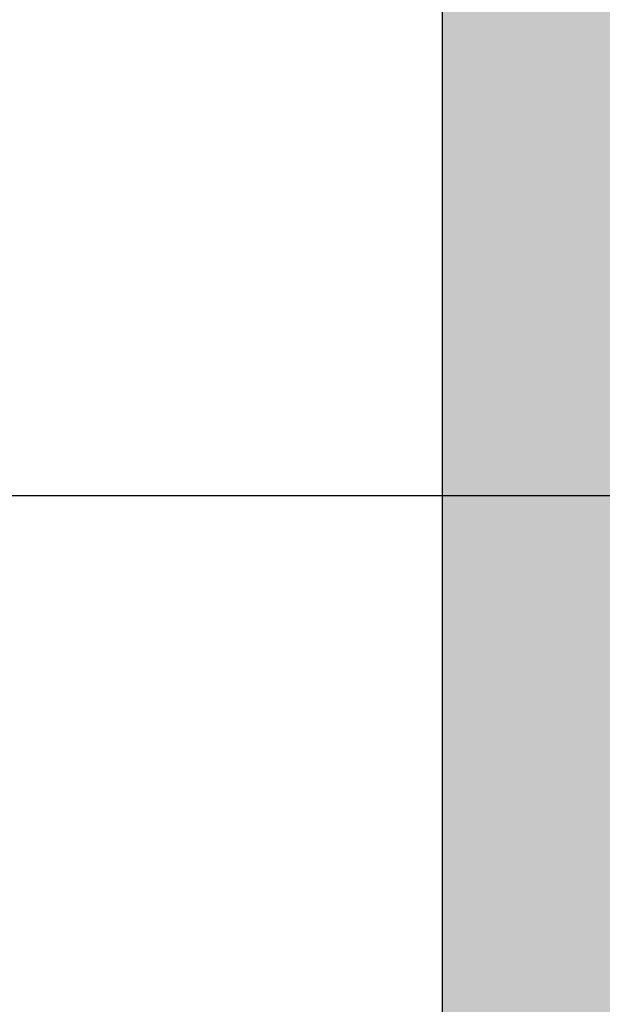
# Model space of a CAD drawing. Units: millimetres. Extents: x -22994 to 29398, y -19990 to 20176.
# Tile 39 of 135: x 190.48 to 197.67, y 41.76 to 53.9. Entities that reach past the tile are written whole.
import ezdxf
from ezdxf import colors
from ezdxf.entities.mleader import LeaderData, LeaderLine
from ezdxf.math import Vec2, Vec3

# ---------------------------------------------------------------- set-up
doc = ezdxf.new("R2010")
doc.units = ezdxf.units.MM
doc.header["$MEASUREMENT"] = 0
for name, color, linetype, lineweight in [('M-ANNO-TEXT', 7, 'Continuous', 25), ('M-DIMS', 2, 'Continuous', 18), ('M-EQPM', 7, 'Continuous', 25), ('M-EQPM-PATT', 7, 'Continuous', 18)]:
    doc.layers.add(name, color=color, linetype=linetype, lineweight=lineweight)
doc.styles.get("Standard").update_dxf_attribs({"font": 'arial.ttf'})
doc.dimstyles.get("Standard").update_dxf_attribs({"dimtxt": 0.18, "dimasz": 10000, "dimexe": 0.18, "dimexo": 0.0625, "dimgap": 0.09, "dimtad": 0, "dimtih": 1, "dimtoh": 1, "dimdec": 0, "dimzin": 0, "dimdsep": 46, "dimtxsty": 'Standard', "dimcen": 0.09, "dimadec": 0, "dimazin": 0, "dimtfac": 1, "dimtdec": 0, "dimtofl": 0, "dimtmove": 0, "dimatfit": 3, "dimfxl": 1, "dimtolj": 1, "dimtzin": 0, "dimlwd": 30, "dimarcsym": 0})

# ---------------------------------------------------------------- blocks, each defined once
blk = doc.blocks.new('*D2')
at = {"layer": 'Defpoints', "color": 0, "transparency": 16777216}
for p in [(6.677, 10.271), (290.852, 10.271), (290.852, -5.079)]:
    blk.add_point(p, dxfattribs=at)
at = {"layer": 'M-DIMS', "color": 0, "lineweight": -2, "transparency": 16777216}
for p, q in [((6.677, 10.209), (6.677, -5.259)), ((290.852, 10.209), (290.852, -5.259))]:
    blk.add_line(p, q, dxfattribs=at)
at = {"layer": 'M-DIMS', "color": 0, "lineweight": 30, "transparency": 16777216}
for p, q in [((-9993.323, -5.079), (-19993.323, -5.079)), ((10290.852, -5.079), (20290.852, -5.079))]:
    blk.add_line(p, q, dxfattribs=at)
at = {"layer": 'M-DIMS', "color": 0, "transparency": 16777216}
for points in [[(-9993.323, 1661.588), (-9993.323, -1671.745), (6.677, -5.079)], [(10290.852, 1661.588), (10290.852, -1671.745), (290.852, -5.079)]]:
    blk.add_solid(points, dxfattribs=at)
at = {"layer": 'M-DIMS', "color": 0, "transparency": 16777216, "insert": (148.765, -5.079), "char_height": 0.18, "attachment_point": 5}
blk.add_mtext('\\A1;284.2', dxfattribs=at)
blk = doc.blocks.new('*D3')
at = {"layer": 'Defpoints', "color": 0, "transparency": 16777216}
for p in [(110.265, 204.165), (110.265, 176.366), (95.833, 127.967)]:
    blk.add_point(p, dxfattribs=at)
at = {"layer": 'M-DIMS', "color": 0, "lineweight": -2, "transparency": 16777216}
for p, q in [((95.833, 128.03), (95.833, 204.345)), ((110.265, 176.429), (110.265, 204.345))]:
    blk.add_line(p, q, dxfattribs=at)
at = {"layer": 'M-DIMS', "color": 0, "lineweight": 30, "transparency": 16777216}
for p, q in [((-9904.167, 204.165), (-19904.167, 204.165)), ((10110.265, 204.165), (20110.265, 204.165))]:
    blk.add_line(p, q, dxfattribs=at)
at = {"layer": 'M-DIMS', "color": 0, "transparency": 16777216}
for points in [[(-9904.167, 1870.832), (-9904.167, -1462.501), (95.833, 204.165)], [(10110.265, 1870.832), (10110.265, -1462.501), (110.265, 204.165)]]:
    blk.add_solid(points, dxfattribs=at)
at = {"layer": 'M-DIMS', "color": 0, "transparency": 16777216, "insert": (103.049, 204.165), "char_height": 0.18, "attachment_point": 5}
blk.add_mtext('\\A1;14.432', dxfattribs=at)
blk = doc.blocks.new('*D4')
at = {"layer": 'Defpoints', "color": 0, "transparency": 16777216}
for p in [(116.265, 204.165), (110.265, 176.366), (116.265, 176.366)]:
    blk.add_point(p, dxfattribs=at)
at = {"layer": 'M-DIMS', "color": 0, "lineweight": -2, "transparency": 16777216}
for p, q in [((110.265, 176.429), (110.265, 204.345)), ((116.265, 176.429), (116.265, 204.345))]:
    blk.add_line(p, q, dxfattribs=at)
at = {"layer": 'M-DIMS', "color": 0, "lineweight": 30, "transparency": 16777216}
for p, q in [((-9889.735, 204.165), (-19889.735, 204.165)), ((10116.265, 204.165), (20116.265, 204.165))]:
    blk.add_line(p, q, dxfattribs=at)
at = {"layer": 'M-DIMS', "color": 0, "transparency": 16777216}
for points in [[(-9889.735, 1870.832), (-9889.735, -1462.501), (110.265, 204.165)], [(10116.265, 1870.832), (10116.265, -1462.501), (116.265, 204.165)]]:
    blk.add_solid(points, dxfattribs=at)
at = {"layer": 'M-DIMS', "color": 0, "transparency": 16777216, "insert": (113.265, 204.165), "char_height": 0.18, "attachment_point": 5}
blk.add_mtext('\\A1;6', dxfattribs=at)
blk = doc.blocks.new('*D5')
at = {"layer": 'Defpoints', "color": 0, "transparency": 16777216}
for p in [(181.265, 204.165), (116.265, 176.366), (181.265, 176.366)]:
    blk.add_point(p, dxfattribs=at)
at = {"layer": 'M-DIMS', "color": 0, "lineweight": -2, "transparency": 16777216}
for p, q in [((116.265, 176.429), (116.265, 204.345)), ((181.265, 176.429), (181.265, 204.345))]:
    blk.add_line(p, q, dxfattribs=at)
at = {"layer": 'M-DIMS', "color": 0, "lineweight": 30, "transparency": 16777216}
for p, q in [((-9883.735, 204.165), (-19883.735, 204.165)), ((10181.265, 204.165), (20181.265, 204.165))]:
    blk.add_line(p, q, dxfattribs=at)
at = {"layer": 'M-DIMS', "color": 0, "transparency": 16777216}
for points in [[(-9883.735, 1870.832), (-9883.735, -1462.501), (116.265, 204.165)], [(10181.265, 1870.832), (10181.265, -1462.501), (181.265, 204.165)]]:
    blk.add_solid(points, dxfattribs=at)
at = {"layer": 'M-DIMS', "color": 0, "transparency": 16777216, "insert": (148.765, 204.165), "char_height": 0.18, "attachment_point": 5}
blk.add_mtext('\\A1;65', dxfattribs=at)
blk = doc.blocks.new('*D6')
at = {"layer": 'Defpoints', "color": 0, "transparency": 16777216}
for p in [(187.265, 204.165), (181.265, 176.366), (187.265, 176.366)]:
    blk.add_point(p, dxfattribs=at)
at = {"layer": 'M-DIMS', "color": 0, "lineweight": -2, "transparency": 16777216}
for p, q in [((181.265, 176.429), (181.265, 204.345)), ((187.265, 176.429), (187.265, 204.345))]:
    blk.add_line(p, q, dxfattribs=at)
at = {"layer": 'M-DIMS', "color": 0, "lineweight": 30, "transparency": 16777216}
for p, q in [((-9818.735, 204.165), (-19818.735, 204.165)), ((10187.265, 204.165), (20187.265, 204.165))]:
    blk.add_line(p, q, dxfattribs=at)
at = {"layer": 'M-DIMS', "color": 0, "transparency": 16777216}
for points in [[(-9818.735, 1870.832), (-9818.735, -1462.501), (181.265, 204.165)], [(10187.265, 1870.832), (10187.265, -1462.501), (187.265, 204.165)]]:
    blk.add_solid(points, dxfattribs=at)
at = {"layer": 'M-DIMS', "color": 0, "transparency": 16777216, "insert": (184.265, 204.165), "char_height": 0.18, "attachment_point": 5}
blk.add_mtext('\\A1;6', dxfattribs=at)
blk = doc.blocks.new('*D7')
at = {"layer": 'Defpoints', "color": 0, "transparency": 16777216}
for p in [(201.697, 204.165), (187.265, 176.366), (201.697, 127.967)]:
    blk.add_point(p, dxfattribs=at)
at = {"layer": 'M-DIMS', "color": 0, "lineweight": -2, "transparency": 16777216}
for p, q in [((187.265, 176.429), (187.265, 204.345)), ((201.697, 128.03), (201.697, 204.345))]:
    blk.add_line(p, q, dxfattribs=at)
at = {"layer": 'M-DIMS', "color": 0, "lineweight": 30, "transparency": 16777216}
for p, q in [((-9812.735, 204.165), (-19812.735, 204.165)), ((10201.697, 204.165), (20201.697, 204.165))]:
    blk.add_line(p, q, dxfattribs=at)
at = {"layer": 'M-DIMS', "color": 0, "transparency": 16777216}
for points in [[(-9812.735, 1870.832), (-9812.735, -1462.501), (187.265, 204.165)], [(10201.697, 1870.832), (10201.697, -1462.501), (201.697, 204.165)]]:
    blk.add_solid(points, dxfattribs=at)
at = {"layer": 'M-DIMS', "color": 0, "transparency": 16777216, "insert": (194.481, 204.165), "char_height": 0.18, "attachment_point": 5}
blk.add_mtext('\\A1;14.432', dxfattribs=at)
blk = doc.blocks.new('*D8')
at = {"layer": 'Defpoints', "color": 0, "transparency": 16777216}
for p in [(227.648, 204.165), (227.648, 146.73), (201.697, 127.967)]:
    blk.add_point(p, dxfattribs=at)
at = {"layer": 'M-DIMS', "color": 0, "lineweight": -2, "transparency": 16777216}
for p, q in [((201.697, 128.03), (201.697, 204.345)), ((227.648, 146.792), (227.648, 204.345))]:
    blk.add_line(p, q, dxfattribs=at)
at = {"layer": 'M-DIMS', "color": 0, "lineweight": 30, "transparency": 16777216}
for p, q in [((-9798.303, 204.165), (-19798.303, 204.165)), ((10227.648, 204.165), (20227.648, 204.165))]:
    blk.add_line(p, q, dxfattribs=at)
at = {"layer": 'M-DIMS', "color": 0, "transparency": 16777216}
for points in [[(-9798.303, 1870.832), (-9798.303, -1462.501), (201.697, 204.165)], [(10227.648, 1870.832), (10227.648, -1462.501), (227.648, 204.165)]]:
    blk.add_solid(points, dxfattribs=at)
at = {"layer": 'M-DIMS', "color": 0, "transparency": 16777216, "insert": (214.673, 204.165), "char_height": 0.18, "attachment_point": 5}
blk.add_mtext('\\A1;25.95', dxfattribs=at)
blk = doc.blocks.new('*D9')
at = {"layer": 'Defpoints', "color": 0, "transparency": 16777216}
for p in [(187.265, 176.366), (306.202, 176.366), (290.852, 10.271)]:
    blk.add_point(p, dxfattribs=at)
at = {"layer": 'M-DIMS', "color": 0, "lineweight": 30, "transparency": 16777216}
for p, q in [((306.202, 10176.366), (306.202, 20176.366)), ((306.202, -9989.729), (306.202, -19989.729))]:
    blk.add_line(p, q, dxfattribs=at)
at = {"layer": 'M-DIMS', "color": 0, "lineweight": -2, "transparency": 16777216}
for p, q in [((187.327, 176.366), (306.382, 176.366)), ((290.915, 10.271), (306.382, 10.271))]:
    blk.add_line(p, q, dxfattribs=at)
at = {"layer": 'M-DIMS', "color": 0, "transparency": 16777216}
for points in [[(-1360.465, 10176.366), (1972.869, 10176.366), (306.202, 176.366)], [(-1360.465, -9989.729), (1972.869, -9989.729), (306.202, 10.271)]]:
    blk.add_solid(points, dxfattribs=at)
at = {"layer": 'M-DIMS', "color": 0, "transparency": 16777216, "insert": (306.202, 93.319), "char_height": 0.18, "attachment_point": 5}
blk.add_mtext('\\A1;166.1', dxfattribs=at)
blk = doc.blocks.new('*D10')
at = {"layer": 'Defpoints', "color": 0, "transparency": 16777216}
for p in [(125.65, 136.071), (133.346, 136.071), (133.346, -5.079)]:
    blk.add_point(p, dxfattribs=at)
at = {"layer": 'M-DIMS', "color": 0, "lineweight": -2, "transparency": 16777216}
for p, q in [((125.65, 136.009), (125.65, -5.259)), ((133.346, 136.009), (133.346, -5.259))]:
    blk.add_line(p, q, dxfattribs=at)
at = {"layer": 'M-DIMS', "color": 0, "lineweight": 30, "transparency": 16777216}
for p, q in [((-9874.35, -5.079), (-19874.35, -5.079)), ((10133.346, -5.079), (20133.346, -5.079))]:
    blk.add_line(p, q, dxfattribs=at)
at = {"layer": 'M-DIMS', "color": 0, "transparency": 16777216}
for points in [[(-9874.35, 1661.588), (-9874.35, -1671.745), (125.65, -5.079)], [(10133.346, 1661.588), (10133.346, -1671.745), (133.346, -5.079)]]:
    blk.add_solid(points, dxfattribs=at)
at = {"layer": 'M-DIMS', "color": 0, "transparency": 16777216, "insert": (129.498, -5.079), "char_height": 0.18, "attachment_point": 5}
blk.add_mtext('\\A1;7.696', dxfattribs=at)
blk = doc.blocks.new('*D11')
at = {"layer": 'Defpoints', "color": 0, "transparency": 16777216}
for p in [(133.346, 136.071), (135.65, 136.071), (135.65, -5.079)]:
    blk.add_point(p, dxfattribs=at)
at = {"layer": 'M-DIMS', "color": 0, "lineweight": -2, "transparency": 16777216}
for p, q in [((133.346, 136.009), (133.346, -5.259)), ((135.65, 136.009), (135.65, -5.259))]:
    blk.add_line(p, q, dxfattribs=at)
at = {"layer": 'M-DIMS', "color": 0, "lineweight": 30, "transparency": 16777216}
for p, q in [((-9866.654, -5.079), (-19866.654, -5.079)), ((10135.65, -5.079), (20135.65, -5.079))]:
    blk.add_line(p, q, dxfattribs=at)
at = {"layer": 'M-DIMS', "color": 0, "transparency": 16777216}
for points in [[(-9866.654, 1661.588), (-9866.654, -1671.745), (133.346, -5.079)], [(10135.65, 1661.588), (10135.65, -1671.745), (135.65, -5.079)]]:
    blk.add_solid(points, dxfattribs=at)
at = {"layer": 'M-DIMS', "color": 0, "transparency": 16777216, "insert": (134.498, -5.079), "char_height": 0.18, "attachment_point": 5}
blk.add_mtext('\\A1;2.304', dxfattribs=at)
blk = doc.blocks.new('*D12')
at = {"layer": 'Defpoints', "color": 0, "transparency": 16777216}
for p in [(135.65, 136.071), (145.65, 136.071), (145.65, -5.079)]:
    blk.add_point(p, dxfattribs=at)
at = {"layer": 'M-DIMS', "color": 0, "lineweight": -2, "transparency": 16777216}
for p, q in [((135.65, 136.009), (135.65, -5.259)), ((145.65, 136.009), (145.65, -5.259))]:
    blk.add_line(p, q, dxfattribs=at)
at = {"layer": 'M-DIMS', "color": 0, "lineweight": 30, "transparency": 16777216}
for p, q in [((-9864.35, -5.079), (-19864.35, -5.079)), ((10145.65, -5.079), (20145.65, -5.079))]:
    blk.add_line(p, q, dxfattribs=at)
at = {"layer": 'M-DIMS', "color": 0, "transparency": 16777216}
for points in [[(-9864.35, 1661.588), (-9864.35, -1671.745), (135.65, -5.079)], [(10145.65, 1661.588), (10145.65, -1671.745), (145.65, -5.079)]]:
    blk.add_solid(points, dxfattribs=at)
at = {"layer": 'M-DIMS', "color": 0, "transparency": 16777216, "insert": (140.65, -5.079), "char_height": 0.18, "attachment_point": 5}
blk.add_mtext('\\A1;10', dxfattribs=at)
blk = doc.blocks.new('*D13')
at = {"layer": 'Defpoints', "color": 0, "transparency": 16777216}
for p in [(145.65, 136.071), (155.65, 136.071), (155.65, -5.079)]:
    blk.add_point(p, dxfattribs=at)
at = {"layer": 'M-DIMS', "color": 0, "lineweight": -2, "transparency": 16777216}
for p, q in [((145.65, 136.009), (145.65, -5.259)), ((155.65, 136.009), (155.65, -5.259))]:
    blk.add_line(p, q, dxfattribs=at)
at = {"layer": 'M-DIMS', "color": 0, "lineweight": 30, "transparency": 16777216}
for p, q in [((-9854.35, -5.079), (-19854.35, -5.079)), ((10155.65, -5.079), (20155.65, -5.079))]:
    blk.add_line(p, q, dxfattribs=at)
at = {"layer": 'M-DIMS', "color": 0, "transparency": 16777216}
for points in [[(-9854.35, 1661.588), (-9854.35, -1671.745), (145.65, -5.079)], [(10155.65, 1661.588), (10155.65, -1671.745), (155.65, -5.079)]]:
    blk.add_solid(points, dxfattribs=at)
at = {"layer": 'M-DIMS', "color": 0, "transparency": 16777216, "insert": (150.65, -5.079), "char_height": 0.18, "attachment_point": 5}
blk.add_mtext('\\A1;10', dxfattribs=at)
blk = doc.blocks.new('*D14')
at = {"layer": 'Defpoints', "color": 0, "transparency": 16777216}
for p in [(155.65, 136.071), (165.65, 136.071), (165.65, -5.079)]:
    blk.add_point(p, dxfattribs=at)
at = {"layer": 'M-DIMS', "color": 0, "lineweight": -2, "transparency": 16777216}
for p, q in [((155.65, 136.009), (155.65, -5.259)), ((165.65, 136.009), (165.65, -5.259))]:
    blk.add_line(p, q, dxfattribs=at)
at = {"layer": 'M-DIMS', "color": 0, "lineweight": 30, "transparency": 16777216}
for p, q in [((-9844.35, -5.079), (-19844.35, -5.079)), ((10165.65, -5.079), (20165.65, -5.079))]:
    blk.add_line(p, q, dxfattribs=at)
at = {"layer": 'M-DIMS', "color": 0, "transparency": 16777216}
for points in [[(-9844.35, 1661.588), (-9844.35, -1671.745), (155.65, -5.079)], [(10165.65, 1661.588), (10165.65, -1671.745), (165.65, -5.079)]]:
    blk.add_solid(points, dxfattribs=at)
at = {"layer": 'M-DIMS', "color": 0, "transparency": 16777216, "insert": (160.65, -5.079), "char_height": 0.18, "attachment_point": 5}
blk.add_mtext('\\A1;10', dxfattribs=at)
blk = doc.blocks.new('*D15')
at = {"layer": 'Defpoints', "color": 0, "transparency": 16777216}
for p in [(173.346, 154.788), (173.346, 136.071), (306.202, 136.071)]:
    blk.add_point(p, dxfattribs=at)
at = {"layer": 'M-DIMS', "color": 0, "lineweight": 30, "transparency": 16777216}
for p, q in [((306.202, 10154.788), (306.202, 20154.788)), ((306.202, -9863.929), (306.202, -19863.929))]:
    blk.add_line(p, q, dxfattribs=at)
at = {"layer": 'M-DIMS', "color": 0, "lineweight": -2, "transparency": 16777216}
for p, q in [((173.408, 154.788), (306.382, 154.788)), ((173.408, 136.071), (306.382, 136.071))]:
    blk.add_line(p, q, dxfattribs=at)
at = {"layer": 'M-DIMS', "color": 0, "transparency": 16777216}
for points in [[(-1360.465, 10154.788), (1972.869, 10154.788), (306.202, 154.788)], [(-1360.465, -9863.929), (1972.869, -9863.929), (306.202, 136.071)]]:
    blk.add_solid(points, dxfattribs=at)
at = {"layer": 'M-DIMS', "color": 0, "transparency": 16777216, "insert": (306.202, 145.43), "char_height": 0.18, "attachment_point": 5}
blk.add_mtext('\\A1;18.717', dxfattribs=at)
blk = doc.blocks.new('*D16')
at = {"layer": 'Defpoints', "color": 0, "transparency": 16777216}
for p in [(120.17, 204.165), (110.466, 48.035), (120.17, 48.035)]:
    blk.add_point(p, dxfattribs=at)
at = {"layer": 'M-DIMS', "color": 0, "lineweight": -2, "transparency": 16777216}
for p, q in [((110.466, 48.097), (110.466, 204.345)), ((120.17, 48.097), (120.17, 204.345))]:
    blk.add_line(p, q, dxfattribs=at)
at = {"layer": 'M-DIMS', "color": 0, "lineweight": 30, "transparency": 16777216}
for p, q in [((-9889.534, 204.165), (-19889.534, 204.165)), ((10120.17, 204.165), (20120.17, 204.165))]:
    blk.add_line(p, q, dxfattribs=at)
at = {"layer": 'M-DIMS', "color": 0, "transparency": 16777216}
for points in [[(-9889.534, 1870.832), (-9889.534, -1462.501), (110.466, 204.165)], [(10120.17, 1870.832), (10120.17, -1462.501), (120.17, 204.165)]]:
    blk.add_solid(points, dxfattribs=at)
at = {"layer": 'M-DIMS', "color": 0, "transparency": 16777216, "insert": (115.318, 204.165), "char_height": 0.18, "attachment_point": 5}
blk.add_mtext('\\A1;9.704', dxfattribs=at)
blk = doc.blocks.new('*D17')
at = {"layer": 'Defpoints', "color": 0, "transparency": 16777216}
for p in [(126.17, 204.165), (120.17, 48.035), (126.17, 48.035)]:
    blk.add_point(p, dxfattribs=at)
at = {"layer": 'M-DIMS', "color": 0, "lineweight": -2, "transparency": 16777216}
for p, q in [((120.17, 48.097), (120.17, 204.345)), ((126.17, 48.097), (126.17, 204.345))]:
    blk.add_line(p, q, dxfattribs=at)
at = {"layer": 'M-DIMS', "color": 0, "lineweight": 30, "transparency": 16777216}
for p, q in [((-9879.83, 204.165), (-19879.83, 204.165)), ((10126.17, 204.165), (20126.17, 204.165))]:
    blk.add_line(p, q, dxfattribs=at)
at = {"layer": 'M-DIMS', "color": 0, "transparency": 16777216}
for points in [[(-9879.83, 1870.832), (-9879.83, -1462.501), (120.17, 204.165)], [(10126.17, 1870.832), (10126.17, -1462.501), (126.17, 204.165)]]:
    blk.add_solid(points, dxfattribs=at)
at = {"layer": 'M-DIMS', "color": 0, "transparency": 16777216, "insert": (123.17, 204.165), "char_height": 0.18, "attachment_point": 5}
blk.add_mtext('\\A1;6', dxfattribs=at)
blk = doc.blocks.new('*D18')
at = {"layer": 'Defpoints', "color": 0, "transparency": 16777216}
for p in [(132.17, 204.165), (126.17, 48.035), (132.17, 48.035)]:
    blk.add_point(p, dxfattribs=at)
at = {"layer": 'M-DIMS', "color": 0, "lineweight": -2, "transparency": 16777216}
for p, q in [((126.17, 48.097), (126.17, 204.345)), ((132.17, 48.097), (132.17, 204.345))]:
    blk.add_line(p, q, dxfattribs=at)
at = {"layer": 'M-DIMS', "color": 0, "lineweight": 30, "transparency": 16777216}
for p, q in [((-9873.83, 204.165), (-19873.83, 204.165)), ((10132.17, 204.165), (20132.17, 204.165))]:
    blk.add_line(p, q, dxfattribs=at)
at = {"layer": 'M-DIMS', "color": 0, "transparency": 16777216}
for points in [[(-9873.83, 1870.832), (-9873.83, -1462.501), (126.17, 204.165)], [(10132.17, 1870.832), (10132.17, -1462.501), (132.17, 204.165)]]:
    blk.add_solid(points, dxfattribs=at)
at = {"layer": 'M-DIMS', "color": 0, "transparency": 16777216, "insert": (129.17, 204.165), "char_height": 0.18, "attachment_point": 5}
blk.add_mtext('\\A1;6', dxfattribs=at)
blk = doc.blocks.new('*D19')
at = {"layer": 'Defpoints', "color": 0, "transparency": 16777216}
for p in [(138.17, 204.165), (132.17, 48.035), (138.17, 48.035)]:
    blk.add_point(p, dxfattribs=at)
at = {"layer": 'M-DIMS', "color": 0, "lineweight": -2, "transparency": 16777216}
for p, q in [((132.17, 48.097), (132.17, 204.345)), ((138.17, 48.097), (138.17, 204.345))]:
    blk.add_line(p, q, dxfattribs=at)
at = {"layer": 'M-DIMS', "color": 0, "lineweight": 30, "transparency": 16777216}
for p, q in [((-9867.83, 204.165), (-19867.83, 204.165)), ((10138.17, 204.165), (20138.17, 204.165))]:
    blk.add_line(p, q, dxfattribs=at)
at = {"layer": 'M-DIMS', "color": 0, "transparency": 16777216}
for points in [[(-9867.83, 1870.832), (-9867.83, -1462.501), (132.17, 204.165)], [(10138.17, 1870.832), (10138.17, -1462.501), (138.17, 204.165)]]:
    blk.add_solid(points, dxfattribs=at)
at = {"layer": 'M-DIMS', "color": 0, "transparency": 16777216, "insert": (135.17, 204.165), "char_height": 0.18, "attachment_point": 5}
blk.add_mtext('\\A1;6', dxfattribs=at)
blk = doc.blocks.new('*D20')
at = {"layer": 'Defpoints', "color": 0, "transparency": 16777216}
for p in [(144.17, 204.165), (138.17, 48.035), (144.17, 48.035)]:
    blk.add_point(p, dxfattribs=at)
at = {"layer": 'M-DIMS', "color": 0, "lineweight": -2, "transparency": 16777216}
for p, q in [((138.17, 48.097), (138.17, 204.345)), ((144.17, 48.097), (144.17, 204.345))]:
    blk.add_line(p, q, dxfattribs=at)
at = {"layer": 'M-DIMS', "color": 0, "lineweight": 30, "transparency": 16777216}
for p, q in [((-9861.83, 204.165), (-19861.83, 204.165)), ((10144.17, 204.165), (20144.17, 204.165))]:
    blk.add_line(p, q, dxfattribs=at)
at = {"layer": 'M-DIMS', "color": 0, "transparency": 16777216}
for points in [[(-9861.83, 1870.832), (-9861.83, -1462.501), (138.17, 204.165)], [(10144.17, 1870.832), (10144.17, -1462.501), (144.17, 204.165)]]:
    blk.add_solid(points, dxfattribs=at)
at = {"layer": 'M-DIMS', "color": 0, "transparency": 16777216, "insert": (141.17, 204.165), "char_height": 0.18, "attachment_point": 5}
blk.add_mtext('\\A1;6', dxfattribs=at)
blk = doc.blocks.new('*D21')
at = {"layer": 'Defpoints', "color": 0, "transparency": 16777216}
for p in [(149.116, 204.165), (144.17, 48.035), (149.116, 48.035)]:
    blk.add_point(p, dxfattribs=at)
at = {"layer": 'M-DIMS', "color": 0, "lineweight": -2, "transparency": 16777216}
for p, q in [((144.17, 48.097), (144.17, 204.345)), ((149.116, 48.097), (149.116, 204.345))]:
    blk.add_line(p, q, dxfattribs=at)
at = {"layer": 'M-DIMS', "color": 0, "lineweight": 30, "transparency": 16777216}
for p, q in [((-9855.83, 204.165), (-19855.83, 204.165)), ((10149.116, 204.165), (20149.116, 204.165))]:
    blk.add_line(p, q, dxfattribs=at)
at = {"layer": 'M-DIMS', "color": 0, "transparency": 16777216}
for points in [[(-9855.83, 1870.832), (-9855.83, -1462.501), (144.17, 204.165)], [(10149.116, 1870.832), (10149.116, -1462.501), (149.116, 204.165)]]:
    blk.add_solid(points, dxfattribs=at)
at = {"layer": 'M-DIMS', "color": 0, "transparency": 16777216, "insert": (146.643, 204.165), "char_height": 0.18, "attachment_point": 5}
blk.add_mtext('\\A1;4.945', dxfattribs=at)
blk = doc.blocks.new('*D22')
at = {"layer": 'Defpoints', "color": 0, "transparency": 16777216}
for p in [(149.116, 30.99), (155.116, 30.99), (155.116, -5.079)]:
    blk.add_point(p, dxfattribs=at)
at = {"layer": 'M-DIMS', "color": 0, "lineweight": -2, "transparency": 16777216}
for p, q in [((149.116, 30.927), (149.116, -5.259)), ((155.116, 30.927), (155.116, -5.259))]:
    blk.add_line(p, q, dxfattribs=at)
at = {"layer": 'M-DIMS', "color": 0, "lineweight": 30, "transparency": 16777216}
for p, q in [((-9850.884, -5.079), (-19850.884, -5.079)), ((10155.116, -5.079), (20155.116, -5.079))]:
    blk.add_line(p, q, dxfattribs=at)
at = {"layer": 'M-DIMS', "color": 0, "transparency": 16777216}
for points in [[(-9850.884, 1661.588), (-9850.884, -1671.745), (149.116, -5.079)], [(10155.116, 1661.588), (10155.116, -1671.745), (155.116, -5.079)]]:
    blk.add_solid(points, dxfattribs=at)
at = {"layer": 'M-DIMS', "color": 0, "transparency": 16777216, "insert": (152.116, -5.079), "char_height": 0.18, "attachment_point": 5}
blk.add_mtext('\\A1;6', dxfattribs=at)
blk = doc.blocks.new('*D23')
at = {"layer": 'Defpoints', "color": 0, "transparency": 16777216}
for p in [(155.116, 30.99), (161.116, 30.99), (161.116, -5.079)]:
    blk.add_point(p, dxfattribs=at)
at = {"layer": 'M-DIMS', "color": 0, "lineweight": -2, "transparency": 16777216}
for p, q in [((155.116, 30.927), (155.116, -5.259)), ((161.116, 30.927), (161.116, -5.259))]:
    blk.add_line(p, q, dxfattribs=at)
at = {"layer": 'M-DIMS', "color": 0, "lineweight": 30, "transparency": 16777216}
for p, q in [((-9844.884, -5.079), (-19844.884, -5.079)), ((10161.116, -5.079), (20161.116, -5.079))]:
    blk.add_line(p, q, dxfattribs=at)
at = {"layer": 'M-DIMS', "color": 0, "transparency": 16777216}
for points in [[(-9844.884, 1661.588), (-9844.884, -1671.745), (155.116, -5.079)], [(10161.116, 1661.588), (10161.116, -1671.745), (161.116, -5.079)]]:
    blk.add_solid(points, dxfattribs=at)
at = {"layer": 'M-DIMS', "color": 0, "transparency": 16777216, "insert": (158.116, -5.079), "char_height": 0.18, "attachment_point": 5}
blk.add_mtext('\\A1;6', dxfattribs=at)
blk = doc.blocks.new('*D24')
at = {"layer": 'Defpoints', "color": 0, "transparency": 16777216}
for p in [(161.116, 30.99), (166.439, 30.99), (166.439, -5.079)]:
    blk.add_point(p, dxfattribs=at)
at = {"layer": 'M-DIMS', "color": 0, "lineweight": -2, "transparency": 16777216}
for p, q in [((161.116, 30.927), (161.116, -5.259)), ((166.439, 30.927), (166.439, -5.259))]:
    blk.add_line(p, q, dxfattribs=at)
at = {"layer": 'M-DIMS', "color": 0, "lineweight": 30, "transparency": 16777216}
for p, q in [((-9838.884, -5.079), (-19838.884, -5.079)), ((10166.439, -5.079), (20166.439, -5.079))]:
    blk.add_line(p, q, dxfattribs=at)
at = {"layer": 'M-DIMS', "color": 0, "transparency": 16777216}
for points in [[(-9838.884, 1661.588), (-9838.884, -1671.745), (161.116, -5.079)], [(10166.439, 1661.588), (10166.439, -1671.745), (166.439, -5.079)]]:
    blk.add_solid(points, dxfattribs=at)
at = {"layer": 'M-DIMS', "color": 0, "transparency": 16777216, "insert": (163.777, -5.079), "char_height": 0.18, "attachment_point": 5}
blk.add_mtext('\\A1;5.323', dxfattribs=at)
blk = doc.blocks.new('*D25')
at = {"layer": 'Defpoints', "color": 0, "transparency": 16777216}
for p in [(166.439, 30.99), (172.439, 30.99), (172.439, -5.079)]:
    blk.add_point(p, dxfattribs=at)
at = {"layer": 'M-DIMS', "color": 0, "lineweight": -2, "transparency": 16777216}
for p, q in [((166.439, 30.927), (166.439, -5.259)), ((172.439, 30.927), (172.439, -5.259))]:
    blk.add_line(p, q, dxfattribs=at)
at = {"layer": 'M-DIMS', "color": 0, "lineweight": 30, "transparency": 16777216}
for p, q in [((-9833.561, -5.079), (-19833.561, -5.079)), ((10172.439, -5.079), (20172.439, -5.079))]:
    blk.add_line(p, q, dxfattribs=at)
at = {"layer": 'M-DIMS', "color": 0, "transparency": 16777216}
for points in [[(-9833.561, 1661.588), (-9833.561, -1671.745), (166.439, -5.079)], [(10172.439, 1661.588), (10172.439, -1671.745), (172.439, -5.079)]]:
    blk.add_solid(points, dxfattribs=at)
at = {"layer": 'M-DIMS', "color": 0, "transparency": 16777216, "insert": (169.439, -5.079), "char_height": 0.18, "attachment_point": 5}
blk.add_mtext('\\A1;6', dxfattribs=at)
blk = doc.blocks.new('*D26')
at = {"layer": 'Defpoints', "color": 0, "transparency": 16777216}
for p in [(172.439, 30.99), (178.439, 30.99), (178.439, -5.079)]:
    blk.add_point(p, dxfattribs=at)
at = {"layer": 'M-DIMS', "color": 0, "lineweight": -2, "transparency": 16777216}
for p, q in [((172.439, 30.927), (172.439, -5.259)), ((178.439, 30.927), (178.439, -5.259))]:
    blk.add_line(p, q, dxfattribs=at)
at = {"layer": 'M-DIMS', "color": 0, "lineweight": 30, "transparency": 16777216}
for p, q in [((-9827.561, -5.079), (-19827.561, -5.079)), ((10178.439, -5.079), (20178.439, -5.079))]:
    blk.add_line(p, q, dxfattribs=at)
at = {"layer": 'M-DIMS', "color": 0, "transparency": 16777216}
for points in [[(-9827.561, 1661.588), (-9827.561, -1671.745), (172.439, -5.079)], [(10178.439, 1661.588), (10178.439, -1671.745), (178.439, -5.079)]]:
    blk.add_solid(points, dxfattribs=at)
at = {"layer": 'M-DIMS', "color": 0, "transparency": 16777216, "insert": (175.439, -5.079), "char_height": 0.18, "attachment_point": 5}
blk.add_mtext('\\A1;6', dxfattribs=at)
blk = doc.blocks.new('*D27')
at = {"layer": 'Defpoints', "color": 0, "transparency": 16777216}
for p in [(178.439, 30.99), (188.117, 30.99), (188.117, -5.079)]:
    blk.add_point(p, dxfattribs=at)
at = {"layer": 'M-DIMS', "color": 0, "lineweight": -2, "transparency": 16777216}
for p, q in [((178.439, 30.927), (178.439, -5.259)), ((188.117, 30.927), (188.117, -5.259))]:
    blk.add_line(p, q, dxfattribs=at)
at = {"layer": 'M-DIMS', "color": 0, "lineweight": 30, "transparency": 16777216}
for p, q in [((-9821.561, -5.079), (-19821.561, -5.079)), ((10188.117, -5.079), (20188.117, -5.079))]:
    blk.add_line(p, q, dxfattribs=at)
at = {"layer": 'M-DIMS', "color": 0, "transparency": 16777216}
for points in [[(-9821.561, 1661.588), (-9821.561, -1671.745), (178.439, -5.079)], [(10188.117, 1661.588), (10188.117, -1671.745), (188.117, -5.079)]]:
    blk.add_solid(points, dxfattribs=at)
at = {"layer": 'M-DIMS', "color": 0, "transparency": 16777216, "insert": (183.278, -5.079), "char_height": 0.18, "attachment_point": 5}
blk.add_mtext('\\A1;9.679', dxfattribs=at)
blk = doc.blocks.new('*D28')
at = {"layer": 'Defpoints', "color": 0, "transparency": 16777216}
for p in [(188.117, 48.035), (306.202, 48.035), (188.117, 30.99)]:
    blk.add_point(p, dxfattribs=at)
at = {"layer": 'M-DIMS', "color": 0, "lineweight": 30, "transparency": 16777216}
for p, q in [((306.202, 10048.035), (306.202, 20048.035)), ((306.202, -9969.01), (306.202, -19969.01))]:
    blk.add_line(p, q, dxfattribs=at)
at = {"layer": 'M-DIMS', "color": 0, "lineweight": -2, "transparency": 16777216}
for p, q in [((188.18, 48.035), (306.382, 48.035)), ((188.18, 30.99), (306.382, 30.99))]:
    blk.add_line(p, q, dxfattribs=at)
at = {"layer": 'M-DIMS', "color": 0, "transparency": 16777216}
for points in [[(-1360.465, 10048.035), (1972.869, 10048.035), (306.202, 48.035)], [(-1360.465, -9969.01), (1972.869, -9969.01), (306.202, 30.99)]]:
    blk.add_solid(points, dxfattribs=at)
at = {"layer": 'M-DIMS', "color": 0, "transparency": 16777216, "insert": (306.202, 39.512), "char_height": 0.18, "attachment_point": 5}
blk.add_mtext('\\A1;17.045', dxfattribs=at)
blk = doc.blocks.new('*D29')
at = {"layer": 'Defpoints', "color": 0, "transparency": 16777216}
for p in [(36.801, 80.045), (64.03, 80.045)]:
    blk.add_point(p, dxfattribs=at)
at = {"layer": 'M-DIMS', "color": 0, "lineweight": -2, "transparency": 16777216}
for p, q in [((50.415, 79.955), (50.415, 80.135)), ((50.325, 80.045), (50.505, 80.045))]:
    blk.add_line(p, q, dxfattribs=at)
at = {"layer": 'M-DIMS', "color": 0, "lineweight": 30, "transparency": 16777216}
blk.add_line((20064.03, 80.03), (10064.03, 80.038), dxfattribs=at)
at = {"layer": 'M-DIMS', "color": 0, "transparency": 16777216}
blk.add_solid([(10064.031, 1746.704), (10064.028, -1586.629), (64.03, 80.045)], dxfattribs=at)
at = {"layer": 'M-DIMS', "color": 0, "transparency": 16777216, "insert": (20064.521, 80.03), "char_height": 0.18, "attachment_point": 5}
blk.add_mtext('\\A1;∅27.23', dxfattribs=at)
blk = doc.blocks.new('*D36')
at = {"layer": 'Defpoints', "color": 0, "transparency": 16777216}
for p in [(46.39, 31.303), (46.387, 26.593)]:
    blk.add_point(p, dxfattribs=at)
at = {"layer": 'M-DIMS', "color": 0, "lineweight": 30, "transparency": 16777216}
for p, q in [((57.15, 20031.301), (51.77, 10031.302)), ((10057.15, 20031.301), (57.15, 20031.301))]:
    blk.add_line(p, q, dxfattribs=at)
at = {"layer": 'M-DIMS', "color": 0, "lineweight": -2, "transparency": 16777216}
for p, q in [((46.389, 28.858), (46.389, 29.038)), ((46.299, 28.948), (46.479, 28.948))]:
    blk.add_line(p, q, dxfattribs=at)
at = {"layer": 'M-DIMS', "color": 0, "transparency": 16777216}
blk.add_solid([(-1614.896, 10032.199), (1718.436, 10030.405), (46.39, 31.303)], dxfattribs=at)
at = {"layer": 'M-DIMS', "color": 0, "transparency": 16777216, "insert": (10057.554, 20031.301), "char_height": 0.18, "attachment_point": 5}
blk.add_mtext('\\A1;∅4.71', dxfattribs=at)
blk = doc.blocks.new('*D37')
at = {"layer": 'Defpoints', "color": 0, "transparency": 16777216}
for p in [(54.834, 118.615), (59.494, 118.614)]:
    blk.add_point(p, dxfattribs=at)
at = {"layer": 'M-DIMS', "color": 0, "lineweight": -2, "transparency": 16777216}
for p, q in [((57.164, 118.524), (57.164, 118.704)), ((57.074, 118.614), (57.254, 118.614))]:
    blk.add_line(p, q, dxfattribs=at)
at = {"layer": 'M-DIMS', "color": 0, "lineweight": 30, "transparency": 16777216}
blk.add_line((20059.493, 116.253), (10059.494, 117.434), dxfattribs=at)
at = {"layer": 'M-DIMS', "color": 0, "transparency": 16777216}
blk.add_solid([(10059.69, 1784.1), (10059.297, -1549.233), (59.494, 118.614)], dxfattribs=at)
at = {"layer": 'M-DIMS', "color": 0, "transparency": 16777216, "insert": (20059.985, 116.253), "char_height": 0.18, "attachment_point": 5}
blk.add_mtext('\\A1;∅4.659', dxfattribs=at)

msp = doc.modelspace()

# ---------------------------------------------------------------- hatches: boundary and pattern name
at = {"layer": 'M-EQPM-PATT'}
h = msp.add_hatch(color=256, dxfattribs=at)
h.set_gradient(color1=(205, 32, 39), color2=(205, 32, 39), tint=1)
h.paths.add_polyline_path([(116.2647, 150.3662), (116.2647, 170.3662), (116.2647, 176.3662), (110.2647, 176.3662), (110.2647, 152.0276), (95.8327, 127.967), (95.8327, 16.6063), (201.6967, 16.6063), (201.6967, 127.967), (187.2647, 152.0276), (187.2647, 176.3662), (181.2647, 176.3662), (181.2647, 170.3662), (181.2647, 150.3662), (195.6967, 126.3055), (195.6967, 22.6063), (101.8327, 22.6063), (101.8327, 126.3055)])
h.paths.add_polyline_path([(185.2208, 88.6347), (101.8327, 88.6347), (101.8327, 87.6347), (182.8066, 87.6347), (178.7313, 83.5594), (195.6967, 83.5594), (195.6967, 84.5594), (181.1455, 84.5594)], flags=17)
h.paths.add_polyline_path([(95.8327, 88.6347), (60.9779, 88.6347, -0.0228552), (61.7178, 87.6347), (95.8327, 87.6347)])
h.paths.add_polyline_path([(215.6212, 86.5189), (215.6212, 80.5999), (220.5095, 83.5594)])
h.paths.add_polyline_path([(215.6212, 84.5594), (201.6967, 84.5594), (201.6967, 83.5594), (215.6212, 83.5594)])
h.paths.add_polyline_path([(225.3978, 86.5189), (220.5095, 83.5594), (225.3978, 80.5999)])
h.paths.add_polyline_path([(231.6256, 84.5594), (225.3978, 84.5594), (225.3978, 83.5594), (231.6256, 83.5594)])

# ---------------------------------------------------------------- linework, layer by layer
at = {"layer": 'M-EQPM'}
msp.add_lwpolyline([(116.2647, 170.3662), (116.2647, 150.3662), (101.8327, 126.3055), (101.8327, 22.6063), (195.6967, 22.6063), (195.6967, 126.3055), (181.2647, 150.3662), (181.2647, 170.3662)], dxfattribs=at)

# ---------------------------------------------------------------- dimensions: what is measured, and where the dimension line sits
at = {"layer": 'M-DIMS'}
for base, p1, p2, override, picture, middle in [((306.202, 176.3662), (290.852, 10.2713), (187.2647, 176.3662), {"dimdec": 1, "dimlfac": 1, "dimrnd": 0, "dimzin": 0, "dimdsep": 46, "dimlunit": 2}, '*D9', (306.202, 93.3187)), ((306.202, 136.0713), (173.3459, 154.788), (173.3459, 136.0713), {"dimdec": 3, "dimlfac": 1, "dimrnd": 0, "dimzin": 0, "dimdsep": 46, "dimlunit": 2}, '*D15', (306.202, 145.4297)), ((306.202, 48.0349), (188.1175, 30.9895), (188.1175, 48.0349), {"dimdec": 3, "dimlfac": 1, "dimrnd": 0, "dimzin": 0, "dimdsep": 46, "dimlunit": 2}, '*D28', (306.202, 39.5122))]:
    dim = msp.add_linear_dim(base=base, p1=p1, p2=p2, angle=90, dimstyle='Standard', override=override, dxfattribs=at)
    dim.commit()
    dim.dimension.update_dxf_attribs({"geometry": picture, "text_midpoint": middle})
dim = msp.add_diameter_dim_2p(p1=(46.3875, 26.5934), p2=(46.39, 31.3035), dimstyle='Standard', override={"dimdec": 2, "dimlfac": 1, "dimrnd": 0, "dimzin": 0, "dimdsep": 46, "dimlunit": 2}, dxfattribs=at)
dim.commit()
dim.dimension.update_dxf_attribs({"geometry": '*D36', "text_midpoint": (10057.5542, 20031.3006), "dimtype": 163})
for base, p1, p2, override, picture, middle in [((110.2647, 204.1654), (95.8327, 127.967), (110.2647, 176.3662), {"dimdec": 3, "dimlfac": 1, "dimrnd": 0, "dimzin": 0, "dimdsep": 46, "dimlunit": 2}, '*D3', (103.0487, 204.1654)), ((116.2647, 204.1654), (110.2647, 176.3662), (116.2647, 176.3662), {"dimdec": 0, "dimlfac": 1, "dimrnd": 0, "dimzin": 0, "dimdsep": 46, "dimlunit": 2}, '*D4', (113.2647, 204.1654)), ((120.1702, 204.1654), (110.4658, 48.0349), (120.1702, 48.0349), {"dimdec": 3, "dimlfac": 1, "dimrnd": 0, "dimzin": 0, "dimdsep": 46, "dimlunit": 2}, '*D16', (115.318, 204.1654)), ((181.2647, 204.1654), (116.2647, 176.3662), (181.2647, 176.3662), {"dimdec": 0, "dimlfac": 1, "dimrnd": 0, "dimzin": 0, "dimdsep": 46, "dimlunit": 2}, '*D5', (148.7647, 204.1654)), ((126.1702, 204.1654), (120.1702, 48.0349), (126.1702, 48.0349), {"dimdec": 0, "dimlfac": 1, "dimrnd": 0, "dimzin": 0, "dimdsep": 46, "dimlunit": 2}, '*D17', (123.1702, 204.1654)), ((132.1702, 204.1654), (126.1702, 48.0349), (132.1702, 48.0349), {"dimdec": 0, "dimlfac": 1, "dimrnd": 0, "dimzin": 0, "dimdsep": 46, "dimlunit": 2}, '*D18', (129.1702, 204.1654)), ((138.1702, 204.1654), (132.1702, 48.0349), (138.1702, 48.0349), {"dimdec": 0, "dimlfac": 1, "dimrnd": 0, "dimzin": 0, "dimdsep": 46, "dimlunit": 2}, '*D19', (135.1702, 204.1654)), ((144.1702, 204.1654), (138.1702, 48.0349), (144.1702, 48.0349), {"dimdec": 0, "dimlfac": 1, "dimrnd": 0, "dimzin": 0, "dimdsep": 46, "dimlunit": 2}, '*D20', (141.1702, 204.1654)), ((149.11567, 204.16539), (144.17023, 48.03494), (149.11567, 48.03494), {"dimdec": 3, "dimlfac": 1, "dimrnd": 0, "dimzin": 0, "dimdsep": 46, "dimlunit": 2}, '*D21', (146.64295, 204.16539)), ((187.2647, 204.1654), (181.2647, 176.3662), (187.2647, 176.3662), {"dimdec": 0, "dimlfac": 1, "dimrnd": 0, "dimzin": 0, "dimdsep": 46, "dimlunit": 2}, '*D6', (184.2647, 204.1654)), ((201.6967, 204.1654), (187.2647, 176.3662), (201.6967, 127.967), {"dimdec": 3, "dimlfac": 1, "dimrnd": 0, "dimzin": 0, "dimdsep": 46, "dimlunit": 2}, '*D7', (194.4807, 204.1654)), ((227.6485, 204.1654), (201.6967, 127.967), (227.6485, 146.7296), {"dimdec": 2, "dimlfac": 1, "dimrnd": 0, "dimzin": 0, "dimdsep": 46, "dimlunit": 2}, '*D8', (214.6726, 204.1654)), ((290.852, -5.0787), (6.6773, 10.2713), (290.852, 10.2713), {"dimdec": 1, "dimlfac": 1, "dimrnd": 0, "dimzin": 0, "dimdsep": 46, "dimlunit": 2}, '*D2', (148.7647, -5.0787)), ((133.3459, -5.0787), (125.6498, 136.0713), (133.3459, 136.0713), {"dimdec": 3, "dimlfac": 1, "dimrnd": 0, "dimzin": 0, "dimdsep": 46, "dimlunit": 2}, '*D10', (129.4978, -5.0787)), ((135.6498, -5.0787), (133.3459, 136.0713), (135.6498, 136.0713), {"dimdec": 3, "dimlfac": 1, "dimrnd": 0, "dimzin": 0, "dimdsep": 46, "dimlunit": 2}, '*D11', (134.4978, -5.0787)), ((145.6498, -5.0787), (135.6498, 136.0713), (145.6498, 136.0713), {"dimdec": 0, "dimlfac": 1, "dimrnd": 0, "dimzin": 0, "dimdsep": 46, "dimlunit": 2}, '*D12', (140.6498, -5.0787)), ((155.6498, -5.0787), (145.6498, 136.0713), (155.6498, 136.0713), {"dimdec": 0, "dimlfac": 1, "dimrnd": 0, "dimzin": 0, "dimdsep": 46, "dimlunit": 2}, '*D13', (150.6498, -5.0787)), ((155.1157, -5.0787), (149.1157, 30.9895), (155.1157, 30.9895), {"dimdec": 0, "dimlfac": 1, "dimrnd": 0, "dimzin": 0, "dimdsep": 46, "dimlunit": 2}, '*D22', (152.1157, -5.0787)), ((161.1157, -5.0787), (155.1157, 30.9895), (161.1157, 30.9895), {"dimdec": 0, "dimlfac": 1, "dimrnd": 0, "dimzin": 0, "dimdsep": 46, "dimlunit": 2}, '*D23', (158.1157, -5.0787)), ((165.6498, -5.0787), (155.6498, 136.0713), (165.6498, 136.0713), {"dimdec": 0, "dimlfac": 1, "dimrnd": 0, "dimzin": 0, "dimdsep": 46, "dimlunit": 2}, '*D14', (160.6498, -5.0787)), ((166.4387, -5.0787), (161.1157, 30.9895), (166.4387, 30.9895), {"dimdec": 3, "dimlfac": 1, "dimrnd": 0, "dimzin": 0, "dimdsep": 46, "dimlunit": 2}, '*D24', (163.7772, -5.0787)), ((172.4387, -5.0787), (166.4387, 30.9895), (172.4387, 30.9895), {"dimdec": 0, "dimlfac": 1, "dimrnd": 0, "dimzin": 0, "dimdsep": 46, "dimlunit": 2}, '*D25', (169.4387, -5.0787)), ((178.4387, -5.0787), (172.4387, 30.9895), (178.4387, 30.9895), {"dimdec": 0, "dimlfac": 1, "dimrnd": 0, "dimzin": 0, "dimdsep": 46, "dimlunit": 2}, '*D26', (175.4387, -5.0787)), ((188.1175, -5.0787), (178.4387, 30.9895), (188.1175, 30.9895), {"dimdec": 3, "dimlfac": 1, "dimrnd": 0, "dimzin": 0, "dimdsep": 46, "dimlunit": 2}, '*D27', (183.2781, -5.0787))]:
    dim = msp.add_linear_dim(base=base, p1=p1, p2=p2, dimstyle='Standard', override=override, dxfattribs=at)
    dim.commit()
    dim.dimension.update_dxf_attribs({"geometry": picture, "text_midpoint": middle})
for p1, p2, override, picture, middle in [((54.8343, 118.6145), (59.4936, 118.614), {"dimdec": 3, "dimlfac": 1, "dimrnd": 0, "dimzin": 0, "dimdsep": 46, "dimlunit": 2}, '*D37', (20059.4934, 116.2531)), ((36.8006, 80.045), (64.0296, 80.045), {"dimdec": 2, "dimlfac": 1, "dimrnd": 0, "dimzin": 0, "dimdsep": 46, "dimlunit": 2}, '*D29', (20064.0296, 80.0303))]:
    dim = msp.add_diameter_dim_2p(p1=p1, p2=p2, dimstyle='Standard', override=override, dxfattribs=at)
    dim.commit()
    dim.dimension.update_dxf_attribs({"geometry": picture, "text_midpoint": middle})

# ---------------------------------------------------------------- leaders
at = {"layer": 'M-ANNO-TEXT'}
ml = msp.add_multileader_mtext('Standard', dxfattribs=at)
ml.set_content('combustion chamber', color=256)
ml.set_leader_properties()
ml.build(insert=Vec2(0, 0))
ml.multileader.update_dxf_attribs({"dogleg_length": 0.36, "arrow_head_size": 200})
ctx = ml.context
ctx.base_point, ctx.char_height, ctx.arrow_head_size, ctx.landing_gap_size, ctx.plane_origin = Vec3(215.7321, 57.9149), 3, 200, 0.09, Vec3(189.1175, 57.9149)
notes = []
notes.append((ctx, [(0, (1, 1, 0), (215.3721, 57.9149), (1, 0), 0.36, [(0, [(189.1175, 57.9149)], 0, [])])]))
ctx.mtext.insert, ctx.mtext.flow_direction = Vec3(215.8221, 59.4394), 5
for ctx, leaders in notes:
    for number, flags, end, landing, length, lines in leaders:
        leader = LeaderData()
        leader.index, (leader.has_last_leader_line, leader.has_dogleg_vector, leader.attachment_direction) = number, flags
        leader.last_leader_point, leader.dogleg_vector, leader.dogleg_length = Vec3(end), Vec3(landing), length
        for number, points, colour, breaks in lines:
            line = LeaderLine()
            line.index, line.vertices, line.color, line.breaks = number, Vec3.list(points), colors.encode_raw_color(colour), breaks
            leader.lines.append(line)
        ctx.leaders.append(leader)

doc.saveas('drawing.dxf')
